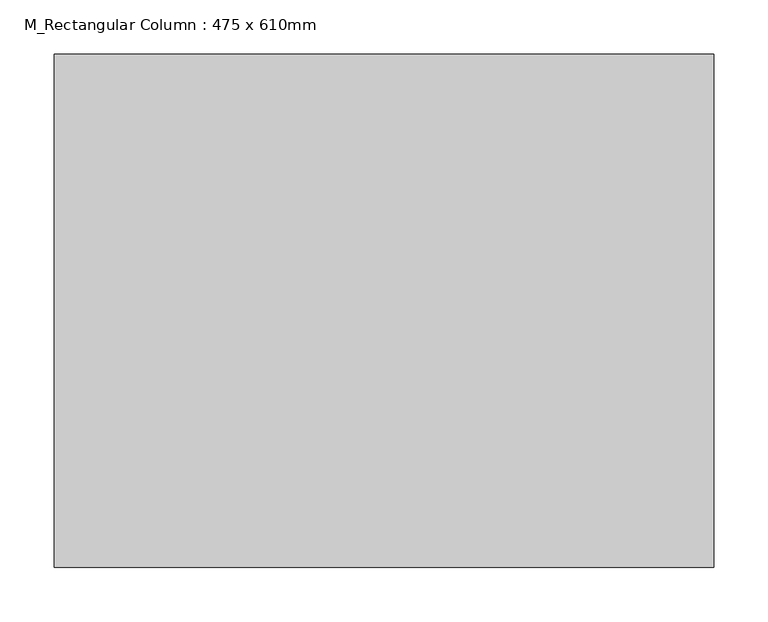
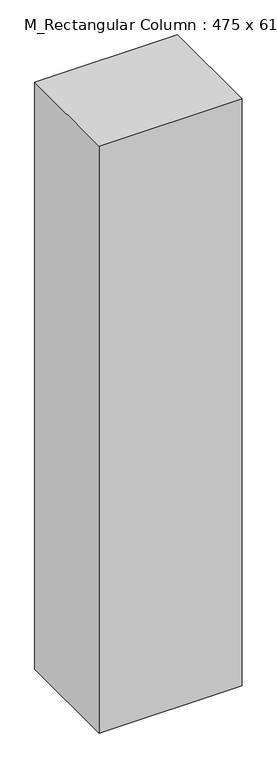
"""IFC4 building model written with IfcOpenShell, lengths in millimetres: column geometry, M_Rectangular Column : 475 x 610mm."""

from ifc_helpers import new_model, si_unit, frame, origin, place, context, project, spatial, polyline, outline, extrude, source, transform, mapped, element, save


def m_rectangular_column_475_x_610mm_ce262976(model_context):
    return source(origin(), model_context, "Body", "SweptSolid", [
        extrude(outline(polyline([(305.0, 237.5), (305.0, -237.5), (-305.0, -237.5), (-305.0, 237.5), (305.0, 237.5)])), frame((0.0, 0.0, 2648.0), z_axis=(0.0, 0.0, 1.0), x_axis=(1.0, 0.0, 0.0)), (0.0, 0.0, 1.0), 2648.0),
    ])


if __name__ == "__main__":
    model = new_model("IFC4")
    model_context = context("Model", 3, world=origin())
    ifc_project = project(units=[si_unit("LENGTHUNIT", "METRE", prefix="MILLI")], contexts=[model_context])
    site = spatial("IfcSite", under=ifc_project)
    building = spatial("IfcBuilding", under=site)
    placement = place(None, origin())
    m_rectangular_column_475_x_610mm_shape = m_rectangular_column_475_x_610mm_ce262976(model_context)
    element("IfcColumn", 1, ObjectType="M_Rectangular Column : 475 x 610mm", at=placement, inside=building, context=model_context, shape_type="MappedRepresentation", body=[
        mapped(m_rectangular_column_475_x_610mm_shape, transform((0.0, 0.0, 0.0), x_axis=(1.0, 0.0, 0.0), y_axis=(0.0, 1.0, 0.0), z_axis=(0.0, 0.0, 1.0))),
    ])
    save(model, "model.ifc")

# Revit data of these elements
# Type "M_Rectangular Column : 475 x 610mm"
#   Depth = 1' - 6.70079"
#   Offset Base = 0' - 0"
#   Offset Top = 0' - 0"
#   Width = 2' - 0.01575"
#   Material = none
